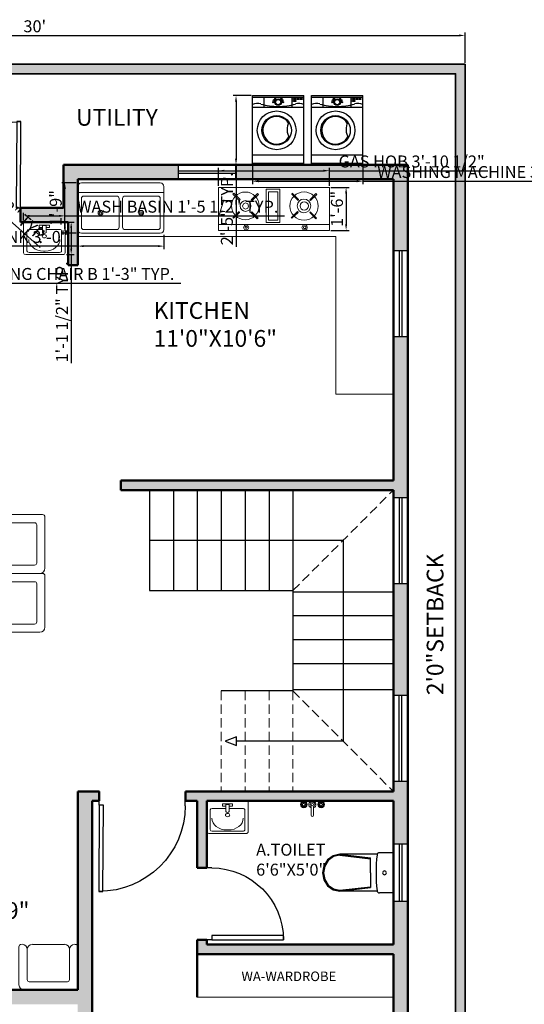
# Model space of a CAD drawing. Units: inches. Extents: x 2638 to 4577, y 1946 to 2619.
# Tile 3 of 8: x 2839 to 3050, y 2207 to 2619. Entities that reach past the tile are written whole.
import ezdxf

# ---------------------------------------------------------------- set-up
doc = ezdxf.new("R2010")
doc.units = ezdxf.units.IN
doc.linetypes.add('DASHED', pattern=[19.05, 12.7, -6.35])
for name, color, linetype, lineweight in [('A-ANNO-DIMS', 2, 'Continuous', 18), ('A-ANNO-TEXT', 7, 'Continuous', 25), ('A-AREA-IDEN', 7, 'Continuous', 25), ('A-DOOR', 4, 'Continuous', 25), ('A-FLOR-FIXT', 8, 'Continuous', 18), ('A-FLOR-OVHD', 8, 'DASHED', 18), ('A-FLOR-STRS', 3, 'Continuous', 25), ('A-FURN', 8, 'Continuous', 18), ('A-GLAZ', 4, 'Continuous', 25), ('A-WALL', 7, 'Continuous', 50), ('A-WALL-PATT', 8, 'Continuous', 13), ('C-PROP', 1, 'Continuous', 35), ('C-PROP-PATT', 252, 'Continuous', 13)]:
    doc.layers.add(name, color=color, linetype=linetype, lineweight=lineweight)
doc.layers.add('SANTEH', color=7, linetype='Continuous')
doc.layers.add('Сантехника', color=7, linetype='Continuous')
doc.styles.get("Standard").update_dxf_attribs({"font": 'arial.ttf'})
doc.dimstyles.new('ISO-25', dxfattribs={"dimtxt": 5, "dimasz": 2.5, "dimexe": 1.25, "dimexo": 0.625, "dimtad": 1, "dimdec": 1, "dimlunit": 3, "dimtxsty": 'Standard', "dimcen": 2.5, "dimclrt": 1, "dimadec": 0, "dimazin": 0, "dimtfac": 1, "dimtdec": 1, "dimtmove": 0, "dimatfit": 3, "dimfxl": 1, "dimarcsym": 0})

# ---------------------------------------------------------------- blocks, each defined once
blk = doc.blocks.new('*D1')
at = {"layer": 'A-ANNO-DIMS', "color": 0, "lineweight": -2, "transparency": 16777216}
for p, q in [((2665.41, 2600.78), (2665.41, 2613.44)), ((2667.91, 2612.19), (3022.91, 2612.19)), ((3025.41, 2600.78), (3025.41, 2613.44))]:
    blk.add_line(p, q, dxfattribs=at)
at = {"layer": 'A-ANNO-DIMS', "color": 0, "transparency": 16777216}
for points in [[(2667.91, 2612.61), (2667.91, 2611.77), (2665.41, 2612.19)], [(3022.91, 2612.61), (3022.91, 2611.77), (3025.41, 2612.19)]]:
    blk.add_solid(points, dxfattribs=at)
at = {"layer": 'Defpoints', "color": 0, "transparency": 16777216}
for p in [(3025.41, 2612.19), (2665.41, 2600.16), (3025.41, 2600.16)]:
    blk.add_point(p, dxfattribs=at)
at = {"layer": 'A-ANNO-DIMS', "color": 0, "transparency": 16777216, "insert": (2845.41, 2615.37), "char_height": 5, "attachment_point": 5}
blk.add_mtext("30'", dxfattribs=at)
blk = doc.blocks.new('*U5')
for p, q in [((0, 0), (0, -6)), ((30, 0), (30, -6))]:
    blk.add_line(p, q)
blk.add_lwpolyline([(0, 0), (0, 30), (1.75, 30), (1.75, 0)], close=True)
blk.add_arc((0, 0), 30, 0, 90)
blk = doc.blocks.new('*U4')
for p, q in [((0, 0), (0, -6)), ((36, 0), (36, -6))]:
    blk.add_line(p, q)
blk.add_lwpolyline([(0, 0), (0, 36), (1.75, 36), (1.75, 0)], close=True)
blk.add_arc((0, 0), 36, 0, 90)
blk = doc.blocks.new('Rac7')
at = {"color": 0}
for p, q in [((-39501, -24232), (-39501, -23830)), ((-39474, -23808), (-38988, -23808)), ((-39457, -23859), (-39457, -24115)), ((-39032, -23838), (-39430, -23838)), ((-39221, -23855), (-39241, -23855)), ((-39005, -24115), (-39005, -23859)), ((-39005, -23859), (-39005, -23859)), ((-38961, -23830), (-38961, -24232)), ((-39253, -24186), (-39253, -24094)), ((-39209, -24186), (-39209, -24094)), ((-38961, -24232), (-39501, -24232)), ((-39430, -24136), (-39253, -24136)), ((-39297, -24164), (-39253, -24164)), ((-39297, -24194), (-39297, -24164)), ((-39165, -24194), (-39297, -24194)), ((-39253, -24186), (-39209, -24186)), ((-39209, -24136), (-39032, -24136)), ((-39209, -24164), (-39165, -24164)), ((-39165, -24164), (-39165, -24194))]:
    blk.add_line(p, q, dxfattribs=at)
at = {"color": 0, "extrusion": (0, 0, -1)}
for centre, major_axis, start_param, end_param in [((-39474, -23830), (-27, 0), 0, 1.570796), ((-39430, -23859), (-27, 0), 0, 1.570796), ((-39241, -24007), (-194, 0), 0, 1.570796), ((-39221, -24007), (-194, 0), 1.570796, 3.141593), ((-39032, -23859), (-27, 0), 1.570796, 3.141593), ((-38988, -23830), (-27, 0), 1.570796, 3.141593), ((-39430, -24115), (-27, 0), -1.570796, 0), ((-39231, -24104), (-25.3, 0), 0.552816, 2.588777), ((-39032, -24115), (-27, 0), -3.141593, -1.570796)]:
    blk.add_ellipse(centre, major_axis=major_axis, ratio=0.785714, start_param=start_param, end_param=end_param, dxfattribs=at)
blk.add_ellipse((-39231, -24048), major_axis=(-27.9, 0), ratio=0.785714, dxfattribs=at)
blk = doc.blocks.new('WC 2 Symb_109')
at = {"layer": 'SANTEH'}
for p, q in [((0, 0), (0, 380)), ((0, 380), (132.4, 380)), ((153.6, 364.9), (506.8, 364.9)), ((506.3, 364.9), (215.7, 330.9)), ((506.3, 356), (215.7, 322)), ((215.7, 190), (215.7, 330.9)), ((215.7, 190), (215.7, 49.1)), ((153.8, 15.1), (506.8, 15.1)), ((506.3, 24), (215.7, 58)), ((506.3, 15.1), (215.7, 49.1)), ((0, 0), (132.4, 0))]:
    blk.add_line(p, q, dxfattribs=at)
for points in [[(154.6, 360.1), (153.9, 364.1), (152.3, 367.9), (150.2, 371.3), (147.4, 374.3), (144.1, 376.7), (140.5, 378.5), (136.5, 379.6), (132.4, 380)], [(154.6, 19.7), (158.6, 62.1), (161.4, 104.7), (163.1, 147.3), (163.7, 189.9), (163.1, 232.5), (161.4, 275.1), (158.6, 317.7), (154.6, 360.1)], [(506.3, 24), (565.5, 36.6), (615.7, 72.6), (649.2, 126.5), (661, 190), (649.2, 253.5), (615.7, 307.4), (565.5, 343.4), (506.3, 356)], [(506.8, 15.1), (569.2, 28.4), (622.2, 66.3), (657.6, 123.1), (670, 190), (657.6, 256.9), (622.2, 313.7), (569.2, 351.6), (506.8, 364.9)], [(132.4, 0), (136.5, 0.4), (140.4, 1.5), (144.1, 3.2), (147.3, 5.6), (150.1, 8.6), (152.3, 12), (153.8, 15.7), (154.6, 19.7)]]:
    blk.add_lwpolyline(points, dxfattribs=at)
blk.add_lwpolyline([(83.6, 208.5), (70.4, 203.1), (64.9, 190), (70.4, 176.9), (83.6, 171.5), (96.8, 176.9), (102.2, 190), (96.8, 203.1)], close=True, dxfattribs=at)
blk = doc.blocks.new('Faucet - Bathroom top')
for p, q in [((-4.107, 0.125), (-4.375, 0.125)), ((-3.75, 0.4788), (-3.75, 0.75)), ((-3.5, 0.482), (-3.5, 0.75)), ((-3.1461, 0.125), (-2.875, 0.125)), ((3.143, 0.125), (2.875, 0.125)), ((3.5, 0.4788), (3.5, 0.75)), ((3.75, 0.482), (3.75, 0.75)), ((4.1039, 0.125), (4.375, 0.125)), ((-4.1039, -0.125), (-4.375, -0.125)), ((-3.75, -0.4821), (-3.75, -0.75)), ((-3.5, -0.4789), (-3.5, -0.75)), ((-3.143, -0.125), (-2.875, -0.125)), ((-0.5, -0.8639), (-0.5, -4.5)), ((0.5, -4.5), (0.5, -0.8631)), ((3.1461, -0.125), (2.875, -0.125)), ((3.5, -0.4821), (3.5, -0.75)), ((3.75, -0.4789), (3.75, -0.75)), ((4.107, -0.125), (4.375, -0.125))]:
    blk.add_line(p, q)
for centre, radius in [((-3.625, 0), 1.375), ((-4.625, 0), 0.2795), ((-3.625, 0), 0.5), ((-3.625, 1), 0.2795), ((-2.625, 0), 0.2795), ((0, 0), 0.5), ((3.625, 0), 1.375), ((2.625, 0), 0.2795), ((3.625, 0), 0.5), ((3.625, 1), 0.2795), ((4.625, 0), 0.2795), ((-3.625, -1), 0.2795), ((3.625, -1), 0.2795)]:
    blk.add_circle(centre, radius)
for centre, radius, start, end in [((-3.625, 0), 1, 105.2407, 164.2093), ((-3.625, 0), 1, 16.44125, 74.07887), ((0, 0), 1.5, 289.6514, 250.3603), ((0, 0), 1, 300.3431, 239.7554), ((3.625, 0), 1, 106.12, 164.0884), ((3.625, 0), 1, 16.23422, 73.90469), ((-3.625, 0), 1, 196.2342, 253.9047), ((-3.625, 0), 1, 286.12, 344.0884), ((3.625, 0), 1, 196.4413, 254.0789), ((3.625, 0), 1, 285.2407, 344.2093), ((0, -4.5), 0.5, 180, 0)]:
    blk.add_arc(centre, radius, start, end)
blk = doc.blocks.new('wash')
at = {"layer": 'Сантехника'}
for p, q in [((4817.13, 2840.92), (4788.24, 2840.92)), ((4788.24, 2819.46), (4788.24, 2840.92)), ((4788.93, 2819.46), (4788.93, 2840.92)), ((4793.08, 2819.46), (4793.08, 2840.92)), ((4812.98, 2819.46), (4812.98, 2840.92)), ((4816.44, 2819.46), (4816.44, 2840.92)), ((4817.13, 2819.46), (4817.13, 2840.92)), ((4793.08, 2836.07), (4788.93, 2836.07)), ((4793.08, 2824.31), (4788.93, 2824.31)), ((4817.13, 2819.46), (4788.24, 2819.46)), ((4817.13, 2816.27), (4788.24, 2816.27)), ((4788.24, 2794.82), (4788.24, 2816.27)), ((4788.93, 2794.82), (4788.93, 2816.27)), ((4793.08, 2794.82), (4793.08, 2816.27)), ((4812.98, 2794.82), (4812.98, 2816.27)), ((4816.44, 2794.82), (4816.44, 2816.27)), ((4817.13, 2794.82), (4817.13, 2816.27)), ((4793.08, 2811.43), (4788.93, 2811.43)), ((4793.08, 2799.66), (4788.93, 2799.66)), ((4817.13, 2794.82), (4788.24, 2794.82))]:
    blk.add_line(p, q, dxfattribs=at)
for points in [[(4789.4, 2839.27), (4789.4, 2840.17), (4789.9, 2840.17), (4789.9, 2839.27)], [(4789.4, 2837.95), (4789.4, 2838.85), (4789.9, 2838.85), (4789.9, 2837.95)], [(4789.4, 2836.64), (4789.4, 2837.53), (4789.9, 2837.53), (4789.9, 2836.64)], [(4790.27, 2836.64), (4790.27, 2837.53), (4790.77, 2837.53), (4790.77, 2836.64)], [(4789.4, 2814.62), (4789.4, 2815.52), (4789.9, 2815.52), (4789.9, 2814.62)], [(4789.4, 2813.31), (4789.4, 2814.2), (4789.9, 2814.2), (4789.9, 2813.31)], [(4789.4, 2811.99), (4789.4, 2812.89), (4789.9, 2812.89), (4789.9, 2811.99)], [(4790.27, 2811.99), (4790.27, 2812.89), (4790.77, 2812.89), (4790.77, 2811.99)]]:
    blk.add_lwpolyline(points, close=True, dxfattribs=at)
for centre, radius in [((4802.77, 2829.54), 8.1), ((4790.19, 2831.93), 0.271), ((4790.98, 2832.18), 0.271), ((4802.77, 2829.54), 6.17), ((4789.46, 2831.45), 0.271), ((4789.46, 2828.92), 0.271), ((4790.98, 2830.19), 1.34), ((4790.98, 2830.19), 1.07), ((4790.19, 2828.4), 0.271), ((4790.98, 2828.15), 0.271), ((4802.77, 2804.9), 8.1), ((4790.19, 2807.28), 0.271), ((4790.98, 2807.53), 0.271), ((4802.77, 2804.9), 6.17), ((4789.46, 2806.8), 0.271), ((4789.46, 2804.27), 0.271), ((4790.98, 2805.55), 1.34), ((4790.98, 2805.55), 1.07), ((4790.19, 2803.75), 0.271), ((4790.98, 2803.5), 0.271)]:
    blk.add_circle(centre, radius, dxfattribs=at)
for centre, radius, start, end in [((4796.44, 2838.85), 4.89, 154.895, 196.6068), ((4762.87, 2829.66), 29.92, 1.0206, 15.0937), ((4802.77, 2829.54), 5.77, 121.8067, 62.1506), ((4802.39, 2840.74), 6.83, 243.19, 300.7673), ((4762.87, 2830.72), 29.92, 344.9063, 358.9794), ((4796.44, 2821.54), 4.89, 163.3932, 205.105), ((4796.44, 2814.2), 4.89, 154.895, 196.6068), ((4762.87, 2805.01), 29.92, 1.0206, 15.0937), ((4802.77, 2804.9), 5.77, 121.8067, 62.1506), ((4802.39, 2816.1), 6.83, 243.19, 300.7673), ((4762.87, 2806.08), 29.92, 344.9063, 358.9794), ((4796.44, 2796.89), 4.89, 163.3932, 205.105)]:
    blk.add_arc(centre, radius, start, end, dxfattribs=at)
blk = doc.blocks.new('Sink-double - 36 in top')
for p, q in [((-18, -4), (18, -4)), ((-0.75, -18.5), (-0.75, -6.5)), ((0.75, -6.5), (0.75, -18.5))]:
    blk.add_line(p, q)
for points in [[(-16.5, 0), (16.5, 0)], [(-18, -19.5), (-18, -1.5)], [(18, -1.5), (18, -19.5)], [(-16.5, -18.5), (-16.5, -6.5)], [(-15.5, -5.5), (-1.75, -5.5)], [(1.75, -5.5), (15.5, -5.5)], [(16.5, -6.5), (16.5, -18.5)], [(-1.75, -19.5), (-15.5, -19.5)], [(15.5, -19.5), (1.75, -19.5)], [(16.5, -21), (-16.5, -21)]]:
    blk.add_lwpolyline(points)
for centre, radius in [((-8.5, -12.5), 1), ((-8.5, -12.5), 0.5), ((8.5, -12.5), 1), ((8.5, -12.5), 0.5)]:
    blk.add_circle(centre, radius)
for centre, radius, start, end in [((-16.5, -1.5), 1.5, 90, 180), ((16.5, -1.5), 1.5, 0, 90), ((-15.5, -6.5), 1, 90, 180), ((-1.75, -6.5), 1, 0, 90), ((1.75, -6.5), 1, 90, 180), ((15.5, -6.5), 1, 0, 90), ((-16.5, -19.5), 1.5, 180, 270), ((-15.5, -18.5), 1, 180, 270), ((-1.75, -18.5), 1, 270, 0), ((1.75, -18.5), 1, 180, 270), ((15.5, -18.5), 1, 270, 0), ((16.5, -19.5), 1.5, 270, 0)]:
    blk.add_arc(centre, radius, start, end)
blk = doc.blocks.new('gas 1')
for points in [[(35.93, -1.87), (35.93, 0), (0, 0), (0, -1.87)], [(8.12, -0.94), (8.44, -1.56), (8.91, -1.87), (9.53, -1.56), (9.84, -0.94), (9.53, -0.31), (8.91, -0.16), (8.44, -0.31)], [(8.59, -0.94), (8.75, -1.25), (8.91, -1.41), (9.22, -1.25), (9.37, -0.94), (9.22, -0.78), (8.91, -0.62), (8.75, -0.78)], [(19.84, -13.28), (15.47, -13.28), (15.47, -2.5), (19.84, -2.5)], [(27.03, -0.94), (27.34, -1.56), (27.97, -1.87), (28.59, -1.56), (28.75, -0.94), (28.59, -0.31), (27.97, -0.16), (27.34, -0.31)], [(27.5, -0.94), (27.65, -1.25), (27.97, -1.41), (28.28, -1.25), (28.28, -0.94), (28.28, -0.62), (27.97, -0.62), (27.65, -0.62)], [(4.84, -3.91), (4.69, -4.06), (6.72, -6.09), (6.87, -5.78)], [(12.81, -3.91), (12.5, -3.75), (10.47, -5.78), (10.78, -5.94)], [(19.22, -12.5), (16.25, -12.5), (16.25, -3.28), (19.22, -3.28)], [(23.75, -3.91), (23.59, -4.06), (25.62, -6.09), (25.78, -5.78)], [(31.71, -3.91), (31.56, -3.75), (29.53, -5.78), (29.68, -5.94)], [(7.81, -7.81), (8.12, -8.59), (8.75, -8.91), (9.53, -8.59), (9.69, -7.81), (9.53, -7.19), (8.75, -6.87), (8.12, -7.19)], [(7.03, -10), (6.72, -9.69), (4.69, -11.72), (5, -12.03)], [(12.97, -11.56), (10.94, -9.69), (10.62, -9.84), (12.65, -11.87)], [(23.75, -11.72), (23.9, -12.03), (25.93, -10), (25.78, -9.69)], [(31.87, -11.56), (29.84, -9.69), (29.53, -9.84), (31.56, -11.87)]]:
    blk.add_lwpolyline(points, close=True)
blk.add_lwpolyline([(35.93, -1.87), (35.93, -13.9), (0, -13.9), (0, -1.87)])
for centre, radius in [((8.7, -7.92), 4.48), ((8.77, -7.89), 1.74), ((27.7, -7.86), 4.58), ((27.69, -7.89), 2.22), ((27.76, -7.89), 1.35)]:
    blk.add_circle(centre, radius)
blk = doc.blocks.new('sofa-27')
at = {"color": 0, "linetype": 'ByBlock'}
for p, q in [((-0.059, 0.059), (-0.059, 0.49)), ((0.035, 0.118), (0.035, 0.461)), ((0.094, 0.52), (0.459, 0.52)), ((0.518, 0.118), (0.518, 0.461)), ((0.613, 0.03), (0.613, 0.49)), ((0.583, 0), (0, 0)), ((0.494, 0.094), (0.059, 0.094))]:
    blk.add_line(p, q, dxfattribs=at)
for centre, radius, start, end in [((-0.03, 0.49), 0.0295, 90, 180), ((-0.024, 0.461), 0.0591, 360, 90), ((0.094, 0.461), 0.0591, 90, 180), ((0.459, 0.461), 0.0591, 0, 90), ((0.577, 0.461), 0.0591, 90, 180), ((0.583, 0.49), 0.0295, 0, 90), ((0.059, 0.118), 0.0236, 180, 270), ((0.494, 0.118), 0.0236, 270, 0), ((0, 0.059), 0.0591, 180, 270), ((0.583, 0.03), 0.0295, 270, 0)]:
    blk.add_arc(centre, radius, start, end, dxfattribs=at)
blk = doc.blocks.new('WIN-36')
for p, q in [((2761.41, 2540.16), (2761.41, 2534.16)), ((2797.41, 2540.16), (2797.41, 2534.16)), ((2761.41, 2537.66), (2797.41, 2537.66)), ((2761.41, 2536.66), (2797.41, 2536.66))]:
    blk.add_line(p, q)
blk = doc.blocks.new('WIN-24')
for p, q in [((2905.41, 2558.16), (2905.41, 2552.16)), ((2929.41, 2558.16), (2929.41, 2552.16)), ((2905.41, 2555.66), (2929.41, 2555.66)), ((2905.41, 2554.66), (2929.41, 2554.66))]:
    blk.add_line(p, q)
blk = doc.blocks.new('*D58')
at = {"layer": 'A-ANNO-DIMS', "color": 0, "lineweight": -2, "transparency": 16777216}
for p, q in [((2792.08, 2568.95), (2794.75, 2571.98)), ((2795.8, 2569.39), (2808.88, 2557.85)), ((2808.91, 2554.11), (2811.58, 2557.14)), ((2810.75, 2556.2), (2847.72, 2523.59))]:
    blk.add_line(p, q, dxfattribs=at)
at = {"layer": 'A-ANNO-DIMS', "color": 0, "transparency": 16777216}
for points in [[(2796.07, 2569.7), (2795.52, 2569.08), (2793.92, 2571.04)], [(2809.15, 2558.16), (2808.6, 2557.54), (2810.75, 2556.2)]]:
    blk.add_solid(points, dxfattribs=at)
at = {"layer": 'Defpoints', "color": 0, "transparency": 16777216}
for p in [(2791.66, 2568.48), (2810.75, 2556.2), (2808.5, 2553.64)]:
    blk.add_point(p, dxfattribs=at)
at = {"layer": 'A-ANNO-DIMS', "color": 1, "transparency": 16777216, "insert": (2832.3, 2541.48), "char_height": 5, "attachment_point": 5, "rotation": 318.5881}
blk.add_mtext('1\'-10 1/2" TYP.', dxfattribs=at)
blk = doc.blocks.new('*D61')
at = {"layer": 'A-ANNO-DIMS', "color": 0, "lineweight": -2, "transparency": 16777216}
for p, q in [((2840.76, 2534.78), (2840.76, 2538)), ((2843.26, 2536.75), (2855.55, 2536.75)), ((2858.05, 2534.78), (2858.05, 2538)), ((2858.05, 2536.75), (2949.94, 2536.75))]:
    blk.add_line(p, q, dxfattribs=at)
at = {"layer": 'A-ANNO-DIMS', "color": 0, "transparency": 16777216}
for points in [[(2843.26, 2537.17), (2843.26, 2536.33), (2840.76, 2536.75)], [(2855.55, 2537.17), (2855.55, 2536.33), (2858.05, 2536.75)]]:
    blk.add_solid(points, dxfattribs=at)
at = {"layer": 'Defpoints', "color": 0, "transparency": 16777216}
for p in [(2858.05, 2536.75), (2840.76, 2534.16), (2858.05, 2534.16)]:
    blk.add_point(p, dxfattribs=at)
at = {"layer": 'A-ANNO-DIMS', "color": 1, "transparency": 16777216, "insert": (2905.25, 2539.96), "char_height": 5, "attachment_point": 5}
blk.add_mtext('WASH BASIN 1\'-5 1/2" TYP.', dxfattribs=at)
blk = doc.blocks.new('*D62')
at = {"layer": 'A-ANNO-DIMS', "color": 0, "lineweight": -2, "transparency": 16777216}
for p, q in [((2858.68, 2534.16), (2861.9, 2534.16)), ((2860.65, 2531.66), (2860.65, 2523.07)), ((2858.68, 2520.57), (2861.9, 2520.57)), ((2860.65, 2520.57), (2860.65, 2475.16))]:
    blk.add_line(p, q, dxfattribs=at)
at = {"layer": 'A-ANNO-DIMS', "color": 0, "transparency": 16777216}
for points in [[(2860.23, 2531.66), (2861.07, 2531.66), (2860.65, 2534.16)], [(2860.23, 2523.07), (2861.07, 2523.07), (2860.65, 2520.57)]]:
    blk.add_solid(points, dxfattribs=at)
at = {"layer": 'Defpoints', "color": 0, "transparency": 16777216}
for p in [(2858.05, 2534.16), (2858.05, 2520.57), (2860.65, 2520.57)]:
    blk.add_point(p, dxfattribs=at)
at = {"layer": 'A-ANNO-DIMS', "color": 1, "transparency": 16777216, "insert": (2857.44, 2496.62), "char_height": 5, "attachment_point": 5, "rotation": 90}
blk.add_mtext('1\'-1 1/2" TYP.', dxfattribs=at)
blk = doc.blocks.new('*D65')
at = {"layer": 'A-ANNO-DIMS', "color": 0, "lineweight": -2, "transparency": 16777216}
for p, q in [((2801.09, 2510.22), (2801.09, 2507.37)), ((2803.59, 2508.62), (2813.43, 2508.62)), ((2815.93, 2510.22), (2815.93, 2507.37)), ((2815.93, 2508.62), (2906.57, 2508.62))]:
    blk.add_line(p, q, dxfattribs=at)
at = {"layer": 'A-ANNO-DIMS', "color": 0, "transparency": 16777216}
for points in [[(2803.59, 2509.04), (2803.59, 2508.21), (2801.09, 2508.62)], [(2813.43, 2509.04), (2813.43, 2508.21), (2815.93, 2508.62)]]:
    blk.add_solid(points, dxfattribs=at)
at = {"layer": 'Defpoints', "color": 0, "transparency": 16777216}
for p in [(2801.09, 2510.85), (2815.93, 2510.85), (2815.93, 2508.62)]:
    blk.add_point(p, dxfattribs=at)
at = {"layer": 'A-ANNO-DIMS', "color": 1, "transparency": 16777216, "insert": (2862.5, 2511.84), "char_height": 5, "attachment_point": 5}
blk.add_mtext('DINING CHAIR B 1\'-3" TYP.', dxfattribs=at)
blk = doc.blocks.new('*D79')
at = {"layer": 'A-ANNO-DIMS', "color": 0, "lineweight": -2, "transparency": 16777216}
for p, q in [((2936.51, 2557.53), (2936.51, 2549.99)), ((2982.61, 2557.53), (2982.61, 2549.99)), ((2939.01, 2551.24), (2980.11, 2551.24)), ((2982.61, 2551.24), (3090.4, 2551.24))]:
    blk.add_line(p, q, dxfattribs=at)
at = {"layer": 'A-ANNO-DIMS', "color": 0, "transparency": 16777216}
for points in [[(2939.01, 2551.66), (2939.01, 2550.82), (2936.51, 2551.24)], [(2980.11, 2551.66), (2980.11, 2550.82), (2982.61, 2551.24)]]:
    blk.add_solid(points, dxfattribs=at)
at = {"layer": 'Defpoints', "color": 0, "transparency": 16777216}
for p in [(2936.51, 2558.16), (2982.61, 2558.16), (2982.61, 2551.24)]:
    blk.add_point(p, dxfattribs=at)
at = {"layer": 'A-ANNO-DIMS', "color": 1, "transparency": 16777216, "insert": (3037.75, 2554.45), "char_height": 5, "attachment_point": 5}
blk.add_mtext('WASHING MACHINE 3\'-10" TYP.', dxfattribs=at)
blk = doc.blocks.new('*D80')
at = {"layer": 'A-ANNO-DIMS', "color": 0, "lineweight": -2, "transparency": 16777216}
for p, q in [((2935.89, 2587.05), (2928.35, 2587.05)), ((2929.6, 2584.55), (2929.6, 2560.66)), ((2935.89, 2558.16), (2928.35, 2558.16)), ((2929.6, 2558.16), (2929.6, 2523.84))]:
    blk.add_line(p, q, dxfattribs=at)
at = {"layer": 'A-ANNO-DIMS', "color": 0, "transparency": 16777216}
for points in [[(2929.18, 2584.55), (2930.02, 2584.55), (2929.6, 2587.05)], [(2929.18, 2560.66), (2930.02, 2560.66), (2929.6, 2558.16)]]:
    blk.add_solid(points, dxfattribs=at)
at = {"layer": 'Defpoints', "color": 0, "transparency": 16777216}
for p in [(2936.51, 2587.05), (2929.6, 2558.16), (2936.51, 2558.16)]:
    blk.add_point(p, dxfattribs=at)
at = {"layer": 'A-ANNO-DIMS', "color": 1, "transparency": 16777216, "insert": (2926.42, 2539.75), "char_height": 5, "attachment_point": 5, "rotation": 90}
blk.add_mtext('2\'-5" TYP.', dxfattribs=at)
blk = doc.blocks.new('*D85')
at = {"layer": 'A-ANNO-DIMS', "color": 0, "lineweight": -2, "transparency": 16777216}
for p, q in [((2863.41, 2528.9), (2863.41, 2522.87)), ((2899.41, 2528.9), (2899.41, 2522.87)), ((2863.41, 2524.12), (2797.71, 2524.12)), ((2896.91, 2524.12), (2865.91, 2524.12))]:
    blk.add_line(p, q, dxfattribs=at)
at = {"layer": 'A-ANNO-DIMS', "color": 0, "transparency": 16777216}
for points in [[(2865.91, 2524.54), (2865.91, 2523.7), (2863.41, 2524.12)], [(2896.91, 2524.54), (2896.91, 2523.7), (2899.41, 2524.12)]]:
    blk.add_solid(points, dxfattribs=at)
at = {"layer": 'Defpoints', "color": 0, "transparency": 16777216}
for p in [(2863.41, 2529.52), (2899.41, 2529.52), (2863.41, 2524.12)]:
    blk.add_point(p, dxfattribs=at)
at = {"layer": 'A-ANNO-DIMS', "color": 1, "transparency": 16777216, "insert": (2829.31, 2527.33), "char_height": 5, "attachment_point": 5}
blk.add_mtext('DOUBLE SINK 3\'-0"', dxfattribs=at)
blk = doc.blocks.new('*D86')
at = {"layer": 'A-ANNO-DIMS', "color": 0, "lineweight": -2, "transparency": 16777216}
for p, q in [((2862.78, 2550.52), (2856.76, 2550.52)), ((2858.01, 2532.02), (2858.01, 2548.02)), ((2862.78, 2529.52), (2856.76, 2529.52))]:
    blk.add_line(p, q, dxfattribs=at)
at = {"layer": 'A-ANNO-DIMS', "color": 0, "transparency": 16777216}
for points in [[(2857.59, 2548.02), (2858.43, 2548.02), (2858.01, 2550.52)], [(2857.59, 2532.02), (2858.43, 2532.02), (2858.01, 2529.52)]]:
    blk.add_solid(points, dxfattribs=at)
at = {"layer": 'Defpoints', "color": 0, "transparency": 16777216}
for p in [(2858.01, 2550.52), (2863.41, 2550.52), (2863.41, 2529.52)]:
    blk.add_point(p, dxfattribs=at)
at = {"layer": 'A-ANNO-DIMS', "color": 1, "transparency": 16777216, "insert": (2854.83, 2540.02), "char_height": 5, "attachment_point": 5, "rotation": 90}
blk.add_mtext('1\'-9"', dxfattribs=at)
blk = doc.blocks.new('*D87')
at = {"layer": 'A-ANNO-DIMS', "color": 0, "lineweight": -2, "transparency": 16777216}
for p, q in [((2922.24, 2549.31), (2922.24, 2556.9)), ((2968.69, 2549.31), (2968.69, 2556.9)), ((2924.74, 2555.65), (2966.19, 2555.65)), ((2968.69, 2555.65), (3034.95, 2555.65))]:
    blk.add_line(p, q, dxfattribs=at)
at = {"layer": 'A-ANNO-DIMS', "color": 0, "transparency": 16777216}
for points in [[(2924.74, 2556.07), (2924.74, 2555.23), (2922.24, 2555.65)], [(2966.19, 2556.07), (2966.19, 2555.23), (2968.69, 2555.65)]]:
    blk.add_solid(points, dxfattribs=at)
at = {"layer": 'Defpoints', "color": 0, "transparency": 16777216}
for p in [(2968.69, 2555.65), (2922.24, 2548.68), (2968.69, 2548.68)]:
    blk.add_point(p, dxfattribs=at)
at = {"layer": 'A-ANNO-DIMS', "color": 1, "transparency": 16777216, "insert": (3003.07, 2558.86), "char_height": 5, "attachment_point": 5}
blk.add_mtext('GAS HOB 3\'-10 1/2"', dxfattribs=at)
blk = doc.blocks.new('*D88')
at = {"layer": 'A-ANNO-DIMS', "color": 0, "lineweight": -2, "transparency": 16777216}
for p, q in [((2969.31, 2548.68), (2976.9, 2548.68)), ((2975.65, 2546.18), (2975.65, 2533.21)), ((2969.31, 2530.71), (2976.9, 2530.71))]:
    blk.add_line(p, q, dxfattribs=at)
at = {"layer": 'A-ANNO-DIMS', "color": 0, "transparency": 16777216}
for points in [[(2975.24, 2546.18), (2976.07, 2546.18), (2975.65, 2548.68)], [(2975.24, 2533.21), (2976.07, 2533.21), (2975.65, 2530.71)]]:
    blk.add_solid(points, dxfattribs=at)
at = {"layer": 'Defpoints', "color": 0, "transparency": 16777216}
for p in [(2968.69, 2548.68), (2968.69, 2530.71), (2975.65, 2530.71)]:
    blk.add_point(p, dxfattribs=at)
at = {"layer": 'A-ANNO-DIMS', "color": 1, "transparency": 16777216, "insert": (2972.47, 2539.7), "char_height": 5, "attachment_point": 5, "rotation": 90}
blk.add_mtext('1\'-6"', dxfattribs=at)

msp = doc.modelspace()

# ---------------------------------------------------------------- hatches: boundary and pattern name
at = {"layer": 'A-WALL-PATT', "transparency": 33554687}
h = msp.add_hatch(color=256, dxfattribs=at)
h.dxf.hatch_style = 1
h.paths.add_polyline_path([(2749.41, 2558.16), (2689.41, 2558.16), (2689.41, 2472.16), (2695.41, 2472.16), (2695.41, 2476.16), (2701.41, 2476.16), (2701.41, 2480.16), (2695.41, 2480.16), (2695.41, 2552.16), (2743.41, 2552.16), (2743.41, 2480.16), (2737.41, 2480.16), (2737.41, 2476.16), (2747.41, 2476.16), (2747.41, 2534.16), (2761.41, 2534.16), (2761.41, 2540.16), (2749.41, 2540.16)])
h.paths.add_polyline_path([(2803.41, 2540.16), (2797.41, 2540.16), (2797.41, 2534.16), (2803.41, 2534.16)])
h.paths.add_polyline_path([(2905.41, 2558.16), (2857.41, 2558.16), (2857.41, 2540.16), (2839.44, 2540.16), (2839.44, 2540.16), (2839.41, 2534.26), (2839.41, 2534.16), (2859.41, 2534.16), (2859.41, 2516.16), (2863.41, 2516.16), (2863.41, 2552.16), (2905.41, 2552.16)])
h.paths.add_polyline_path([(3001.41, 2558.16), (2929.41, 2558.16), (2929.41, 2552.16), (2995.41, 2552.16), (2995.41, 2522.16), (3001.41, 2522.16)])
h.paths.add_polyline_path([(3001.41, 2486.16), (2995.41, 2486.16), (2995.41, 2426.16), (2881.41, 2426.16), (2881.41, 2422.16), (2995.41, 2422.16), (2995.41, 2418.91), (3001.41, 2418.91)])
h.paths.add_polyline_path([(3001.41, 2382.91), (2995.41, 2382.91), (2995.41, 2336.41), (3001.41, 2336.41)])
h.paths.add_polyline_path([(3001.41, 2300.41), (2995.41, 2300.41), (2995.41, 2296.16), (2908.41, 2296.16), (2908.41, 2292.16), (2913.41, 2292.16), (2913.41, 2264.16), (2917.41, 2264.16), (2917.41, 2292.16), (2995.41, 2292.16), (2995.41, 2274.16), (3001.41, 2274.16)])
h.paths.add_polyline_path([(3001.41, 2250.16), (2995.41, 2250.16), (2995.41, 2232.16), (2917.41, 2232.16), (2917.41, 2234.16), (2913.41, 2234.16), (2913.41, 2228.16), (2995.41, 2228.16), (2995.41, 2096.16), (3001.41, 2096.16)])
h.paths.add_polyline_path([(3001.41, 2060.16), (2995.41, 2060.16), (2995.41, 2024.16), (2971.41, 2024.16), (2971.41, 2018.16), (3001.41, 2018.16)])
h.paths.add_polyline_path([(2869.41, 2292.16), (2872.41, 2292.16), (2872.41, 2296.16), (2863.41, 2296.16), (2863.41, 2213.16), (2833.41, 2213.16), (2833.41, 2207.16), (2863.41, 2207.16), (2863.41, 2018.16), (2893.41, 2018.16), (2893.41, 2024.16), (2869.41, 2024.16)])
h.paths.add_polyline_path([(2809.41, 2213.16), (2767.41, 2213.16), (2767.41, 2216.16), (2761.41, 2216.16), (2761.41, 2207.16), (2809.41, 2207.16)])
h.paths.add_polyline_path([(2671.41, 2290.16), (2761.41, 2290.16), (2761.41, 2288.16), (2767.41, 2288.16), (2767.41, 2290.16), (2791.41, 2290.16), (2791.41, 2296.16), (2695.41, 2296.16), (2695.41, 2320.16), (2689.41, 2320.16), (2689.41, 2296.16), (2665.41, 2296.16), (2665.41, 2193.16), (2671.41, 2193.16)])
h.paths.add_polyline_path([(2695.41, 2448.16), (2689.41, 2448.16), (2689.41, 2404.16), (2695.41, 2404.16)])
at = {"layer": 'C-PROP-PATT', "transparency": 33554687}
h = msp.add_hatch(color=256, dxfattribs=at)
h.dxf.hatch_style = 1
h.paths.add_polyline_path([(3025.41, 2600.16), (2665.41, 2600.16), (2665.41, 2296.16), (2669.41, 2296.16), (2669.41, 2596.16), (3021.41, 2596.16), (3021.41, 2004.16), (2863.41, 2004.16), (2863.41, 2000.16), (3025.41, 2000.16)])
h.paths.add_polyline_path([(2669.41, 2193.16), (2665.41, 2193.16), (2665.41, 2000.16), (2669.41, 2000.16)], flags=17)

# ---------------------------------------------------------------- linework, layer by layer
at = {"layer": 'A-FLOR-FIXT'}
for p, q in [((2863.41, 2528.16), (2971.41, 2528.16)), ((2971.41, 2528.16), (2971.41, 2462.16)), ((2971.41, 2462.16), (2995.41, 2462.16))]:
    msp.add_line(p, q, dxfattribs=at)
at = {"layer": 'A-FLOR-OVHD', "ltscale": 0.3}
for p, q in [((2953.41, 2380.16), (2995.41, 2422.16)), ((2923.41, 2338.16), (2923.41, 2296.16)), ((2933.41, 2338.16), (2933.41, 2296.16)), ((2943.41, 2338.16), (2943.41, 2296.16)), ((2953.41, 2338.16), (2953.41, 2296.16)), ((2953.41, 2338.16), (2995.41, 2296.16))]:
    msp.add_line(p, q, dxfattribs=at)
at = {"layer": 'A-FLOR-STRS'}
for p, q in [((2893.41, 2422.16), (2893.41, 2380.16)), ((2903.41, 2422.16), (2903.41, 2380.16)), ((2913.41, 2422.16), (2913.41, 2380.16)), ((2923.41, 2422.16), (2923.41, 2380.16)), ((2933.41, 2422.16), (2933.41, 2380.16)), ((2943.41, 2422.16), (2943.41, 2380.16)), ((2953.41, 2422.16), (2953.41, 2338.16)), ((2893.41, 2380.16), (2953.41, 2380.16)), ((2953.41, 2379.66), (2995.41, 2379.66)), ((2953.41, 2369.66), (2995.41, 2369.66)), ((2953.41, 2359.66), (2995.41, 2359.66)), ((2953.41, 2349.66), (2995.41, 2349.66)), ((2953.41, 2338.16), (2923.41, 2338.16)), ((2995.41, 2338.66), (2953.41, 2338.66))]:
    msp.add_line(p, q, dxfattribs=at)
msp.add_lwpolyline([(2893.41, 2401.16), (2974.41, 2401.16), (2974.41, 2317.16), (2929.8, 2317.16)], dxfattribs=at)
msp.add_lwpolyline([(2925.03, 2317.16), (2929.8, 2315.29), (2929.8, 2319.03)], close=True, dxfattribs=at)
at = {"layer": 'A-FURN'}
msp.add_line((2995.41, 2210.16), (2913.41, 2210.16), dxfattribs=at)
at = {"layer": 'A-WALL'}
for p, q in [((2857.41, 2558.16), (2857.41, 2540.16)), ((2857.41, 2558.16), (3001.41, 2558.16)), ((3001.41, 2558.16), (3001.41, 2018.16)), ((2863.41, 2552.16), (2863.41, 2516.16)), ((2863.41, 2552.16), (2995.41, 2552.16)), ((2995.41, 2552.16), (2995.41, 2426.16)), ((2839.41, 2540.16), (2839.41, 2534.16)), ((2839.41, 2540.16), (2857.41, 2540.16)), ((2839.41, 2534.16), (2859.41, 2534.16)), ((2859.41, 2534.16), (2859.41, 2516.16)), ((2859.41, 2516.16), (2863.41, 2516.16)), ((2881.41, 2426.16), (2995.41, 2426.16)), ((2881.41, 2426.16), (2881.41, 2422.16)), ((2881.41, 2422.16), (2995.41, 2422.16)), ((2995.41, 2422.16), (2995.41, 2296.16)), ((2863.41, 2296.16), (2863.41, 2213.16)), ((2872.41, 2296.16), (2863.41, 2296.16)), ((2872.41, 2296.16), (2872.41, 2292.16)), ((2995.41, 2296.16), (2908.41, 2296.16)), ((2908.41, 2296.16), (2908.41, 2292.16)), ((2869.41, 2292.16), (2869.41, 2024.16)), ((2872.41, 2292.16), (2869.41, 2292.16)), ((2913.41, 2292.16), (2908.41, 2292.16)), ((2913.41, 2292.16), (2913.41, 2264.16)), ((2995.41, 2292.16), (2917.41, 2292.16)), ((2917.41, 2292.16), (2917.41, 2264.16)), ((2995.41, 2292.16), (2995.41, 2232.16)), ((2917.41, 2264.16), (2913.41, 2264.16)), ((2917.41, 2234.16), (2913.41, 2234.16)), ((2913.41, 2234.16), (2913.41, 2210.16)), ((2917.41, 2234.16), (2917.41, 2232.16)), ((2995.41, 2232.16), (2917.41, 2232.16)), ((2995.41, 2228.16), (2913.41, 2228.16)), ((2995.41, 2228.16), (2995.41, 2024.16)), ((2863.41, 2213.16), (2767.41, 2213.16))]:
    msp.add_line(p, q, dxfattribs=at)
at = {"layer": 'C-PROP'}
for points in [[(2669.41, 2000.16), (2665.41, 2000.16), (2665.41, 2600.16), (3025.41, 2600.16), (3025.41, 2000.16), (2863.41, 2000.16)], [(2669.41, 2296.16), (2669.41, 2596.16), (3021.41, 2596.16), (3021.41, 2004.16), (2863.41, 2004.16)]]:
    msp.add_lwpolyline(points, dxfattribs=at)

# ---------------------------------------------------------------- block references
at = {"layer": 'A-DOOR', "xscale": -1}
for name, p, rotation in [('*U4', (2839.44, 2540.16), 359.6786649249896), ('*U4', (2872.38, 2290.36), 179.6786649249896), ('*U5', (2919.41, 2234.16), 270)]:
    msp.add_blockref(name, p, dxfattribs=dict(at, rotation=rotation))
at = {"layer": 'A-FLOR-FIXT', "rotation": 270}
msp.add_blockref('wash', (141.7, 7375.29), dxfattribs=at)
at = {"layer": 'A-FLOR-FIXT', "xscale": -1}
msp.add_blockref('Sink-double - 36 in top', (2881.41, 2550.52), dxfattribs=at)
at = {"layer": 'A-FLOR-FIXT', "rotation": 180}
for name, p, xscale, yscale, zscale in [('gas 1', (2922.24, 2530.71), -1.292580420916565, 1.292580420916565, 1.292580420916565), ('Rac7', (4107.43, 1757.1), -0.0320670790485951, 0.0320670790485951, 0.0320670790485951), ('Rac7', (4184.08, 1515.1), -0.0320670790485951, 0.0320670790485951, 0.0320670790485951), ('WC 2 Symb_109', (2995.41, 2270.55), 0.0441898926459964, 0.0441898926459964, 0.0441898926459964)]:
    msp.add_blockref(name, p, dxfattribs=dict(at, xscale=xscale, yscale=yscale, zscale=zscale))
at = {"layer": 'A-FLOR-FIXT'}
msp.add_blockref('Faucet - Bathroom top', (2961.55, 2290.66), dxfattribs=at)
at = {"layer": 'A-FURN', "xscale": 36.66436083614781, "yscale": 36.66436083614781, "zscale": 36.66436083614781, "rotation": 90}
for p in [(2849.68, 2389.46), (2849.68, 2364.84)]:
    msp.add_blockref('sofa-27', p, dxfattribs=at)
at = {"layer": 'A-FURN', "xscale": 36.66436083614781, "yscale": 36.66436083614781, "zscale": 36.66436083614781}
msp.add_blockref('sofa-27', (2840.95, 2213.16), dxfattribs=at)
at = {"layer": 'A-GLAZ'}
msp.add_blockref('WIN-24', (0, 0), dxfattribs=at)
for name, p, rotation in [('WIN-36', (461.25, 5283.57), 270.0000000000056), ('WIN-36', (461.25, 5180.32), 270.0000000000059), ('WIN-36', (5535.57, -461), 90.00000000000254), ('WIN-24', (443.25, 5179.57), 270.0000000000061)]:
    msp.add_blockref(name, p, dxfattribs=dict(at, rotation=rotation))

# ---------------------------------------------------------------- texts
at = {"layer": 'A-ANNO-TEXT', "attachment_point": 1}
for s, width, insert, char_height in [('{\\fTimes New Roman|b0|i0|c0|p18;UTILITY}', 61.0557, (2862.71, 2581.44), 7), ('WA-WARDROBE', 29.5334, (2931.87, 2220.86), 4)]:
    msp.add_mtext_dynamic_manual_height_columns(s, width=width, gutter_width=12.5, heights=[0], dxfattribs=dict(at, insert=insert, char_height=char_height))
at = {"layer": 'A-ANNO-TEXT', "insert": (3009.37, 2336.4), "char_height": 7, "attachment_point": 1, "rotation": 90}
msp.add_mtext_dynamic_manual_height_columns('{\\fTimes New Roman|b0|i0|c0|p18;2\'0"SETBACK}', width=61.0557, gutter_width=12.5, heights=[0], dxfattribs=at)
at = {"layer": 'A-AREA-IDEN', "attachment_point": 1}
for s, insert, char_height in [('{\\fTimes New Roman|b0|i0|c0|p18;KITCHEN\\P11\'0"X10\'6"}', (2895.11, 2500.7), 7), ('{\\fTimes New Roman|b0|i0|c0|p18;A.TOILET\\P6\'6"X5\'0"}', (2938.02, 2274.28), 5), ('{\\fTimes New Roman|b0|i0|c0|p18;FOYER\\P8\'0"X6\'9"}', (2802.15, 2261.53), 7)]:
    msp.add_mtext_dynamic_manual_height_columns(s, width=61.0557, gutter_width=12.5, heights=[0], dxfattribs=dict(at, insert=insert, char_height=char_height))

# ---------------------------------------------------------------- dimensions: what is measured, and where the dimension line sits
at = {"layer": 'A-ANNO-DIMS'}
dim = msp.add_linear_dim(base=(3025.41, 2612.19), p1=(2665.41, 2600.16), p2=(3025.41, 2600.16), dimstyle='ISO-25', override={"dimclrd": 0, "dimclre": 0, "dimclrt": 0}, dxfattribs=at)
dim.commit()
dim.dimension.update_dxf_attribs({"geometry": '*D1', "text_midpoint": (2845.41, 2615.37)})
for base, p1, p2, angle, text, picture, middle in [((2929.6, 2558.16), (2936.51, 2587.05), (2936.51, 2558.16), 270, '<> TYP.', '*D80', (2926.42, 2539.75)), ((2810.75, 2556.2), (2791.66, 2568.48), (2808.5, 2553.64), 318.5881, '<> TYP.', '*D58', (2832.3, 2541.48)), ((2863.41, 2524.12), (2899.41, 2529.52), (2863.41, 2529.52), 180, 'DOUBLE SINK <>', '*D85', (2829.31, 2527.33)), ((2860.65, 2520.57), (2858.05, 2534.16), (2858.05, 2520.57), 270, '<> TYP.', '*D62', (2857.44, 2496.62))]:
    dim = msp.add_linear_dim(base=base, p1=p1, p2=p2, angle=angle, text=text, dimstyle='ISO-25', override={"dimdec": 1, "dimrnd": 0, "dimzin": 1, "dimlunit": 4, "dimfrac": 2}, dxfattribs=at)
    dim.commit()
    dim.dimension.update_dxf_attribs({"geometry": picture, "text_midpoint": middle})
for base, p1, p2, text, picture, middle in [((2968.6859, 2555.649), (2922.2393, 2548.6821), (2968.6859, 2548.6821), 'GAS HOB <>', '*D87', (3003.0677, 2558.8627)), ((2982.61, 2551.24), (2936.51, 2558.16), (2982.61, 2558.16), 'WASHING MACHINE <> TYP.', '*D79', (3037.75, 2554.45)), ((2858.05, 2536.75), (2840.76, 2534.16), (2858.05, 2534.16), 'WASH BASIN <> TYP.', '*D61', (2905.25, 2539.96)), ((2815.93, 2508.62), (2801.09, 2510.85), (2815.93, 2510.85), 'DINING CHAIR B <> TYP.', '*D65', (2862.5, 2511.84))]:
    dim = msp.add_linear_dim(base=base, p1=p1, p2=p2, text=text, dimstyle='ISO-25', override={"dimdec": 1, "dimrnd": 0, "dimzin": 1, "dimlunit": 4, "dimfrac": 2}, dxfattribs=at)
    dim.commit()
    dim.dimension.update_dxf_attribs({"geometry": picture, "text_midpoint": middle})
for base, p1, p2, angle, picture, middle in [((2858.01, 2550.52), (2863.41, 2529.52), (2863.41, 2550.52), 90, '*D86', (2854.83, 2540.02)), ((2975.65, 2530.71), (2968.69, 2548.68), (2968.69, 2530.71), 270, '*D88', (2972.47, 2539.7))]:
    dim = msp.add_linear_dim(base=base, p1=p1, p2=p2, angle=angle, dimstyle='ISO-25', override={"dimdec": 1, "dimrnd": 0, "dimzin": 1, "dimlunit": 4, "dimfrac": 2}, dxfattribs=at)
    dim.commit()
    dim.dimension.update_dxf_attribs({"geometry": picture, "text_midpoint": middle})

doc.saveas('drawing.dxf')
